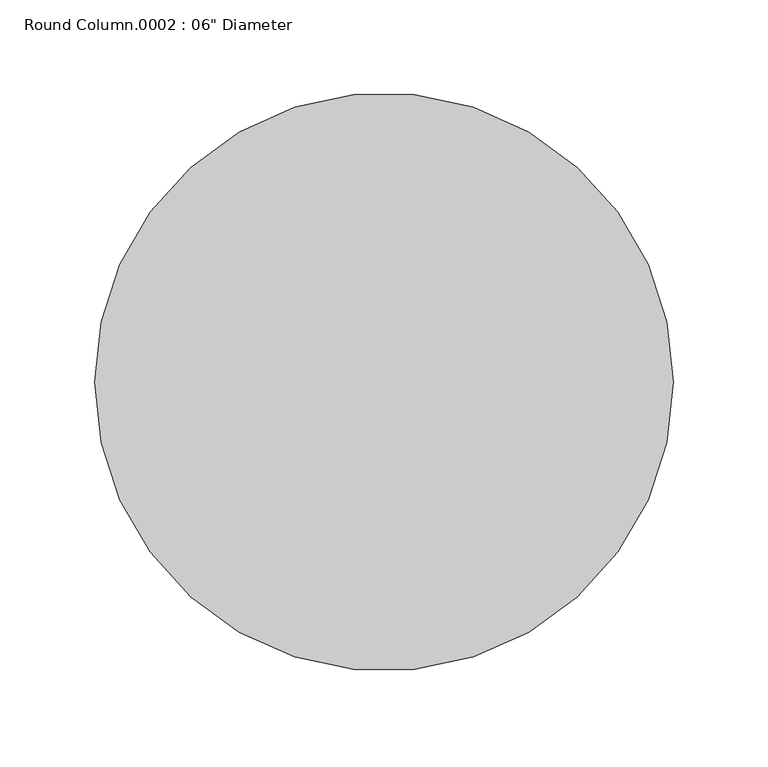
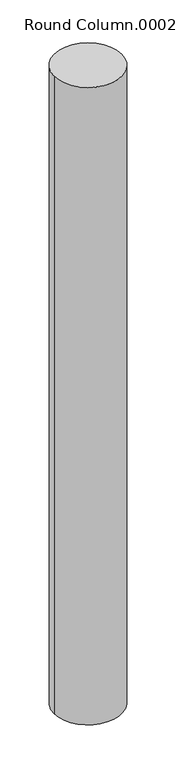
"""IFC4 building model written with IfcOpenShell, lengths in millimetres: column geometry."""

from ifc_helpers import new_model, si_unit, point, frame, frame_2d, origin, place, context, project, spatial, circle_curve, trimmed, segment, composite_curve, outline, extrude, source, transform, mapped, element, save


def column_6a8e800d(model_context):
    return source(origin(), model_context, "Body", "SweptSolid", [
        extrude(outline(composite_curve([segment(trimmed(circle_curve(frame_2d((3997.9193638, 6851.4883261)), 152.4), [point((3845.5193638, 6851.4883261))], [point((4150.3193638, 6851.4883261))], False, "CARTESIAN"), True, "CONTINUOUS"), segment(trimmed(circle_curve(frame_2d((3997.9193638, 6851.4883261)), 152.4), [point((4150.3193638, 6851.4883261))], [point((3845.5193638, 6851.4883261))], False, "CARTESIAN"), True, "CONTINUOUS")], self_intersect=False)), frame((0.0, 0.0, 6553.2), z_axis=(0.0, 0.0, 1.0), x_axis=(1.0, 0.0, 0.0)), (0.0, 0.0, 1.0), 3048.0),
    ])


if __name__ == "__main__":
    model = new_model("IFC4")
    model_context = context("Model", 3, world=origin())
    ifc_project = project(units=[si_unit("LENGTHUNIT", "METRE", prefix="MILLI")], contexts=[model_context])
    site = spatial("IfcSite", under=ifc_project)
    building = spatial("IfcBuilding", under=site)
    placement = place(None, origin())
    column_shape = column_6a8e800d(model_context)
    element("IfcColumn", 1, ObjectType="Round Column.0002 : 06\" Diameter", at=placement, inside=building, context=model_context, shape_type="MappedRepresentation", body=[
        mapped(column_shape, transform((0.0, 0.0, 0.0), x_axis=(1.0, 0.0, 0.0), y_axis=(0.0, 1.0, 0.0), z_axis=(0.0, 0.0, 1.0))),
    ])
    save(model, "model.ifc")

# Revit data of these elements
# Type "Round Column.0002 : 06\" Diameter"
#   Assembly Code = "B1010200"
#   Diameter = 0' - 6"
#   Offset Base = 0' - 0"
#   Offset Top = 0' - 0"
#   Material = none
